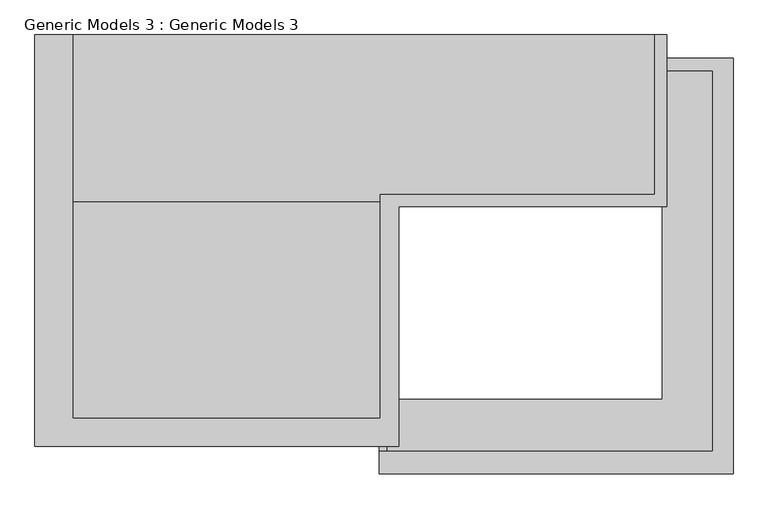
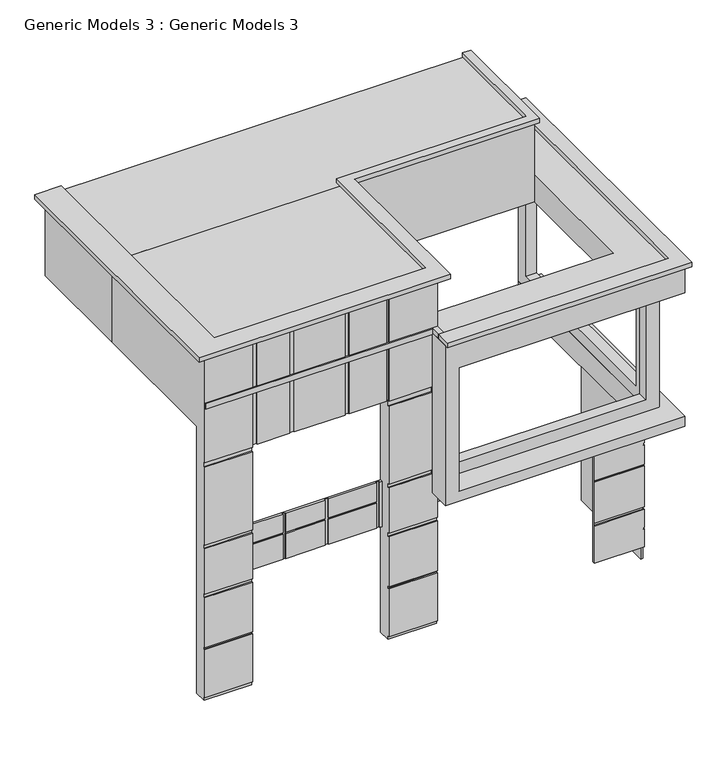
"""IFC4 building model written with IfcOpenShell, lengths in millimetres: proxy geometry, Generic Models 3 : Generic Models 3."""

from ifc_helpers import new_model, si_unit, frame, origin, place, context, project, spatial, polyline, outline, extrude, faceted_brep, source, transform, mapped, element, save


def generic_models_3_generic_models_3_1ac72cdd(model_context):
    return source(origin(), model_context, "Body", "SolidModel", [
        faceted_brep([(-5562.3530968, -13017.658307, 304.8), (-5562.3530968, -12966.858307, 304.8), (-5562.3530968, -12966.858307, 0.0), (-5562.3530968, -12279.4426078, 0.0), (-5562.3530968, -12279.4426078, 707.2361937), (-5562.3530968, -13017.658307, 707.2361937), (-5562.3530968, -13017.658307, 2147.6565444), (-5562.3530968, -13017.658307, 1217.4178641), (-5562.3530968, -12242.958307, 1217.4178641), (-5562.3530968, -12242.958307, 2148.7323728), (-5562.3530968, -12992.258307, 2148.7323728), (-5562.3530968, -12992.258307, 2147.6565444), (-5562.3530968, -12992.258307, 1150.8363185), (-5562.3530968, -13017.658307, 1150.8363185), (-5562.3530968, -13017.658307, 744.9879539), (-5562.3530968, -12242.958307, 744.9879539), (-5562.3530968, -12242.958307, 1148.7718933), (-5562.3530968, -12992.258307, 1148.7718933), (-5562.3530968, -11633.358307, 2630.7756431), (-5562.3530968, -11633.358307, 2189.781496), (-5562.3530968, -10744.358307, 2189.781496), (-5562.3530968, -10744.358307, 2630.7756431), (-5562.3530968, -11633.358307, 1148.7718933), (-5562.3530968, -11633.358307, 744.9879539), (-5562.3530968, -10744.358307, 744.9879539), (-5562.3530968, -10744.358307, 1148.7718933), (-5562.3530968, -11633.358307, 2148.7323728), (-5562.3530968, -11633.358307, 1217.4178641), (-5562.3530968, -10744.358307, 1217.4178641), (-5562.3530968, -10744.358307, 2148.7323728), (-5562.3530968, -12242.958307, 2189.781496), (-5562.3530968, -12242.958307, 2630.7756431), (-5562.3530968, -13017.658307, 2630.7756431), (-5562.3530968, -13017.658307, 2189.781496), (-5562.3530968, -10744.358307, 0.0), (-5562.3530968, -10744.358307, 707.2361937), (-5562.3530968, -11584.7454289, 707.2361937), (-5562.3530968, -11584.7454289, 0.0), (-5562.3530968, -10744.358307, 2670.8659469), (-5562.3530968, -10744.358307, 3048.0), (-5562.3530968, -11633.358307, 3048.0), (-5562.3530968, -11633.358307, 2670.8659469), (-5562.3530968, -13017.658307, 3048.0), (-5562.3530968, -13017.658307, 2670.8659469), (-5562.3530968, -12242.958307, 2670.8659469), (-5562.3530968, -12242.958307, 3048.0), (-5562.3530968, -12242.958307, 0.0), (-5562.3530968, -11633.358307, 0.0), (-5562.3530968, -11633.358307, 707.2361937), (-5562.3530968, -12242.958307, 707.2361937), (-5562.3530968, -11672.0594166, 3048.0), (-5562.3530968, -12209.5923832, 3048.0), (-5562.3530968, -12209.5923832, 2670.8659469), (-5562.3530968, -11672.0594166, 2670.8659469), (-5613.1530968, -12966.858307, 3048.0), (-5613.1530968, -10744.358307, 3048.0), (-5613.1530968, -10744.358307, 0.0), (-5613.1530968, -12966.858307, 0.0), (-5613.1530968, -12966.858307, 304.8), (-5613.1530968, -11633.358307, 2630.7756431), (-5613.1530968, -12242.958307, 2630.7756431), (-5613.1530968, -12242.958307, 744.9879539), (-5613.1530968, -11633.358307, 744.9879539), (-5587.7530968, -11584.7454289, 0.0), (-5587.7530968, -11633.358307, 0.0), (-5587.7530968, -12242.958307, 0.0), (-5587.7530968, -12279.4426078, 0.0), (-5587.7530968, -12242.958307, 2630.7756431), (-5587.7530968, -12242.958307, 2189.781496), (-5587.7530968, -12242.958307, 2148.7323728), (-5587.7530968, -12242.958307, 1217.4178641), (-5587.7530968, -12242.958307, 1148.7718933), (-5587.7530968, -12242.958307, 744.9879539), (-6641.8530968, -12966.858307, 3048.0), (-6641.8530968, -13017.658307, 3048.0), (-5587.7530968, -12242.958307, 3048.0), (-5587.7530968, -12209.5923832, 3048.0), (-5587.7530968, -11672.0594166, 3048.0), (-5587.7530968, -11633.358307, 3048.0), (-5587.7530968, -11633.358307, 2630.7756431), (-5587.7530968, -10744.358307, 2670.8659469), (-5587.7530968, -10744.358307, 2630.7756431), (-5587.7530968, -10744.358307, 2189.781496), (-5587.7530968, -10744.358307, 2148.7323728), (-5587.7530968, -10744.358307, 1217.4178641), (-5587.7530968, -10744.358307, 1148.7718933), (-5587.7530968, -10744.358307, 744.9879539), (-5587.7530968, -10744.358307, 707.2361937), (-5587.7530968, -11633.358307, 744.9879539), (-5587.7530968, -11633.358307, 1148.7718933), (-5587.7530968, -11633.358307, 1217.4178641), (-5587.7530968, -11633.358307, 2148.7323728), (-5587.7530968, -11633.358307, 2189.781496), (-6641.8530968, -13017.658307, 2189.781496), (-5587.7530968, -13017.658307, 2630.7756431), (-5587.7530968, -13017.658307, 2670.8659469), (-6641.8530968, -13017.658307, 304.8), (-5587.7530968, -13017.658307, 707.2361937), (-5587.7530968, -13017.658307, 744.9879539), (-6641.8530968, -13017.658307, 1150.8363185), (-6641.8530968, -13017.658307, 2147.6565444), (-6641.8530968, -13017.658307, 1217.4178641), (-6641.8530968, -12966.858307, 304.8), (-6641.8530968, -12992.258307, 1150.8363185), (-6641.8530968, -12992.258307, 1217.4178641), (-6641.8530968, -12992.258307, 2147.6565444), (-6641.8530968, -12992.258307, 2189.781496), (-5587.7530968, -12992.258307, 1150.8363185), (-5587.7530968, -12992.258307, 1217.4178641), (-5587.7530968, -12992.258307, 2148.7323728), (-5587.7530968, -12992.258307, 2189.781496), (-5587.7530968, -12992.258307, 1148.7718933), (-5587.7530968, -12279.4426078, 707.2361937), (-5587.7530968, -12242.958307, 707.2361937), (-5587.7530968, -11633.358307, 707.2361937), (-5587.7530968, -11584.7454289, 707.2361937), (-5587.7530968, -11672.0594166, 2670.8659469), (-5587.7530968, -12209.5923832, 2670.8659469), (-5587.7530968, -12242.958307, 2670.8659469), (-5587.7530968, -11633.358307, 2670.8659469)], [[[0, 1, 2, 3, 4, 5]], [[6, 7, 8, 9, 10, 11]], [[12, 13, 14, 15, 16, 17]], [[18, 19, 20, 21]], [[22, 23, 24, 25]], [[26, 27, 28, 29]], [[30, 31, 32, 33]], [[34, 35, 36, 37]], [[38, 39, 40, 41]], [[42, 43, 44, 45]], [[46, 47, 48, 49]], [[50, 51, 52, 53]], [[54, 55, 56, 57, 58], [59, 60, 61, 62]], [[57, 2, 1, 58]], [[2, 57, 56, 34, 37, 63, 64, 47, 46, 65, 66, 3]], [[61, 60, 67, 31, 30, 68, 69, 9, 8, 70, 71, 16, 15, 72]], [[55, 54, 73, 74, 42, 45, 75, 76, 51, 50, 77, 78, 40, 39]], [[60, 59, 79, 67]], [[55, 39, 38, 80, 81, 21, 20, 82, 83, 29, 28, 84, 85, 25, 24, 86, 87, 35, 34, 56]], [[59, 62, 88, 23, 22, 89, 90, 27, 26, 91, 92, 19, 18, 79]], [[62, 61, 72, 88]], [[42, 74, 93, 33, 32, 94, 95, 43]], [[96, 0, 5, 97, 98, 14, 13, 99]], [[100, 101, 7, 6]], [[102, 73, 54, 58]], [[73, 102, 96, 99, 103, 104, 101, 100, 105, 106, 93, 74]], [[0, 96, 102, 58, 1]], [[104, 103, 107, 108]], [[105, 11, 10, 109, 110, 106]], [[11, 105, 100, 6]], [[33, 93, 106, 110, 68, 30]], [[13, 12, 107, 103, 99]], [[7, 101, 104, 108, 70, 8]], [[68, 110, 109, 69]], [[70, 108, 107, 111, 71]], [[82, 92, 91, 83]], [[84, 90, 89, 85]], [[72, 98, 97, 112, 66, 65, 113, 114, 64, 63, 115, 87, 86, 88]], [[77, 116, 117, 76, 75, 118, 95, 94, 67, 79, 81, 80, 119, 78]], [[69, 109, 10, 9]], [[71, 111, 17, 16]], [[17, 111, 107, 12]], [[83, 91, 26, 29]], [[92, 82, 20, 19]], [[85, 89, 22, 25]], [[90, 84, 28, 27]], [[49, 48, 114, 113]], [[35, 87, 115, 36]], [[97, 5, 4, 112]], [[98, 72, 15, 14]], [[88, 86, 24, 23]], [[53, 52, 117, 116]], [[80, 38, 41, 119]], [[43, 95, 118, 44]], [[67, 94, 32, 31]], [[81, 79, 18, 21]], [[113, 65, 46, 49]], [[66, 112, 4, 3]], [[115, 63, 37, 36]], [[64, 114, 48, 47]], [[76, 117, 52, 51]], [[118, 75, 45, 44]], [[78, 119, 41, 40]], [[116, 77, 50, 53]]]),
        extrude(outline(polyline([(-10299.4530968, -13297.058307), (-15214.3530968, -13297.058307), (-15214.3530968, -13271.658307), (-10299.4530968, -13271.658307), (-10299.4530968, -13297.058307)])), frame((0.0, 0.0, 6988.8180197), z_axis=(0.0, 0.0, 1.0), x_axis=(1.0, 0.0, 0.0)), (0.0, 0.0, 1.0), 123.1819803),
        extrude(outline(polyline([(-5016.2530968, -13845.289875), (-10299.4530968, -13845.289875), (-10299.4530968, -13513.2632996), (-5320.7863052, -13513.2632996), (-5320.7863052, -7825.1949722), (-6070.3530968, -7825.1949722), (-6070.3530968, -7641.8252058), (-5016.2530968, -7641.8252058), (-5016.2530968, -13845.289875)])), frame((0.0, 0.0, 7010.4), z_axis=(0.0, 0.0, 1.0), x_axis=(1.0, 0.0, 0.0)), (0.0, 0.0, 1.0), 101.6),
        extrude(outline(polyline([(-10185.1530968, -13513.2632996), (-10299.4530968, -13513.2632996), (-10299.4530968, -13271.658307), (-10185.1530968, -13271.658307), (-10185.1530968, -13513.2632996)])), frame((0.0, 0.0, 7010.4), z_axis=(0.0, 0.0, 1.0), x_axis=(1.0, 0.0, 0.0)), (0.0, 0.0, 1.0), 101.6),
        extrude(outline(polyline([(-15436.9164492, -7289.958307), (-14871.4530968, -7289.958307), (-14871.4530968, -13017.658307), (-10285.554919, -13017.658307), (-10285.554919, -9672.4992532), (-6185.8200713, -9672.4992532), (-6185.8200713, -7289.958307), (-6006.8530968, -7289.958307), (-6006.8530968, -9854.918289), (-10002.8085028, -9854.918289), (-10002.8085028, -13437.0410181), (-15436.9164492, -13437.0410181), (-15436.9164492, -7289.958307)])), frame((0.0, 0.0, 8229.6), z_axis=(0.0, 0.0, 1.0), x_axis=(1.0, 0.0, 0.0)), (0.0, 0.0, 1.0), 101.6),
        extrude(outline(polyline([(-6070.3530968, -9781.0408857), (-15214.3530968, -9781.0408857), (-15214.3530968, -7289.958307), (-6070.3530968, -7289.958307), (-6070.3530968, -9781.0408857)])), frame((0.0, 0.0, 6400.8), z_axis=(0.0, 0.0, 1.0), x_axis=(1.0, 0.0, 0.0)), (0.0, 0.0, 1.0), 1828.8),
        faceted_brep([(-5384.1292606, -13043.058307, 6400.8), (-5384.1292606, -13043.058307, 3581.4), (-5384.5530968, -13043.058307, 3581.4), (-5384.5530968, -13043.058307, 6400.8), (-10002.8085028, -13043.058307, 3581.4), (-10002.8085028, -13043.058307, 6400.8), (-5613.1530968, -13043.058307, 6400.8), (-5613.1530968, -13043.058307, 3581.4), (-5676.6530968, -13043.058307, 3851.8605085), (-5676.6530968, -13043.058307, 6146.8), (-9740.6530968, -13043.058307, 6146.8), (-9740.6530968, -13043.058307, 3851.8605085), (-5384.1292606, -13271.658307, 6400.8), (-10002.8085028, -13271.658307, 6400.8), (-10002.8085028, -13271.658307, 3581.4), (-5384.1292606, -13271.658307, 3581.4), (-5676.6530968, -13271.658307, 6146.8), (-5676.6530968, -13271.658307, 3851.8605085), (-9740.6530968, -13271.658307, 3851.8605085), (-9740.6530968, -13271.658307, 6146.8), (-5613.1530968, -8394.858307, 3581.4), (-5384.5530968, -8394.858307, 3581.4), (-5384.5530968, -8394.858307, 6400.8), (-5613.1530968, -8394.858307, 6400.8), (-5384.5530968, -8674.258307, 6146.8), (-5384.5530968, -8674.258307, 3860.8), (-5384.5530968, -12789.058307, 3860.8), (-5384.5530968, -12789.058307, 6146.8), (-5613.1530968, -8674.258307, 3860.8), (-5613.1530968, -8674.258307, 6146.8), (-5613.1530968, -12789.058307, 6146.8), (-5613.1530968, -12789.058307, 3860.8)], [[[0, 1, 2, 3]], [[4, 5, 6, 7], [8, 9, 10, 11]], [[12, 13, 14, 15], [16, 17, 18, 19]], [[1, 0, 12, 15]], [[15, 14, 4, 7, 20, 21, 2, 1]], [[5, 4, 14, 13]], [[13, 12, 0, 3, 22, 23, 6, 5]], [[16, 9, 8, 17]], [[17, 8, 11, 18]], [[18, 11, 10, 19]], [[9, 16, 19, 10]], [[22, 3, 2, 21], [24, 25, 26, 27]], [[23, 20, 7, 6], [28, 29, 30, 31]], [[22, 21, 20, 23]], [[24, 29, 28, 25]], [[25, 28, 31, 26]], [[26, 31, 30, 27]], [[29, 24, 27, 30]]]),
        faceted_brep([(-5117.8530968, -8394.858307, 3581.4), (-5613.1530968, -8394.858307, 3581.4), (-5613.1530968, -12966.858307, 3581.4), (-10299.4530968, -12966.858307, 3581.4), (-10299.4530968, -13271.658307, 3581.4), (-10002.8085028, -13271.658307, 3581.4), (-10002.8085028, -13766.185809, 3581.4), (-5117.8530968, -13766.185809, 3581.4), (-5117.8530968, -13766.185809, 3352.8), (-10299.4530968, -13766.185809, 3352.8), (-10299.4530968, -12966.858307, 3352.8), (-10185.1530968, -12966.858307, 3352.8), (-10185.1530968, -13195.458307, 3352.8), (-5384.5530968, -13195.458307, 3352.8), (-5384.5530968, -8394.858307, 3352.8), (-5117.8530968, -8394.858307, 3352.8), (-5613.1530968, -12966.858307, 3048.0), (-10185.1530968, -12966.858307, 3048.0), (-10299.4530968, -13766.185809, 7010.4), (-10299.4530968, -13271.658307, 7010.4), (-10002.8085028, -13766.185809, 6400.8), (-5117.8530968, -13766.185809, 6400.8), (-5117.8530968, -13766.185809, 7010.4), (-5384.5530968, -8394.858307, 3048.0), (-5613.1530968, -8394.858307, 3048.0), (-5384.5530968, -13195.458307, 3048.0), (-10185.1530968, -13195.458307, 3048.0), (-5117.8530968, -7709.058307, 7010.4), (-6070.3530968, -7709.058307, 7010.4), (-6070.3530968, -12738.258307, 7010.4), (-10185.1530968, -12738.258307, 7010.4), (-10185.1530968, -13271.658307, 7010.4), (-10185.1530968, -13271.658307, 6400.8), (-10002.8085028, -13271.658307, 6400.8), (-10185.1530968, -12738.258307, 6400.8), (-6070.3530968, -12738.258307, 6400.8), (-6070.3530968, -7709.058307, 6400.8), (-5117.8530968, -7709.058307, 6400.8)], [[[0, 1, 2, 3, 4, 5, 6, 7]], [[8, 9, 10, 11, 12, 13, 14, 15]], [[7, 8, 15, 0]], [[10, 3, 2, 16, 17, 11]], [[10, 9, 18, 19, 4, 3]], [[9, 8, 7, 6, 20, 21, 22, 18]], [[1, 0, 15, 14, 23, 24]], [[2, 1, 24, 16]], [[23, 14, 13, 25]], [[16, 24, 23, 25, 26, 17]], [[12, 26, 25, 13]], [[26, 12, 11, 17]], [[19, 18, 22, 27, 28, 29, 30, 31]], [[4, 19, 31, 32, 33, 5]], [[6, 5, 33, 20]], [[21, 20, 33, 32, 34, 35, 36, 37]], [[27, 22, 21, 37]], [[34, 30, 29, 35]], [[30, 34, 32, 31]], [[28, 27, 37, 36]], [[29, 28, 36, 35]]]),
        faceted_brep([(-15214.3530968, -13271.658307, 8229.6), (-15214.3530968, -13271.658307, 5748.0360394), (-14185.6530968, -13271.658307, 5748.0360394), (-14185.6530968, -13271.658307, 8229.6), (-14082.3684215, -13271.658307, 5780.2418911), (-13378.2700012, -13271.658307, 5780.2418911), (-13378.2700012, -13271.658307, 8229.6), (-14082.3684215, -13271.658307, 8229.6), (-13280.9266618, -13271.658307, 5780.2418911), (-12184.1917045, -13271.658307, 5780.2418911), (-12184.1917045, -13271.658307, 8229.6), (-13280.9266618, -13271.658307, 8229.6), (-12099.827477, -13271.658307, 5780.2418911), (-11290.0530968, -13271.658307, 5780.2418911), (-11290.0530968, -13271.658307, 8229.6), (-12099.827477, -13271.658307, 8229.6), (-10185.1530968, -13271.658307, 8229.6), (-11233.851605, -13271.658307, 8229.6), (-11233.851605, -13271.658307, 5767.0860394), (-10299.4530968, -13271.658307, 5767.0860394), (-10299.4530968, -13271.658307, 5646.4360394), (-11233.851605, -13271.658307, 5646.4360394), (-11233.851605, -13271.658307, 3866.4235575), (-10299.4530968, -13271.658307, 3866.4235575), (-10299.4530968, -13271.658307, 3783.7672722), (-11233.851605, -13271.658307, 3783.7672722), (-11233.851605, -13271.658307, 2744.8217298), (-10185.1530968, -13271.658307, 2744.8217298), (-14185.6530968, -13271.658307, 5646.4360394), (-15214.3530968, -13271.658307, 5646.4360394), (-15214.3530968, -13271.658307, 3866.4235575), (-14185.6530968, -13271.658307, 3866.4235575), (-14185.6530968, -13271.658307, 2744.8217298), (-14185.6530968, -13271.658307, 3783.7672722), (-15214.3530968, -13271.658307, 3783.7672722), (-15214.3530968, -13271.658307, 2744.8217298), (-14185.6530968, -13271.658307, 1524.8108649), (-14185.6530968, -13271.658307, 2666.5766837), (-15214.3530968, -13271.658307, 2666.5766837), (-15214.3530968, -13271.658307, 1524.8108649), (-14185.6530968, -13271.658307, 382.6097323), (-14185.6530968, -13271.658307, 1479.6035006), (-15214.3530968, -13271.658307, 1479.6035006), (-15214.3530968, -13271.658307, 382.6097323), (-10185.1530968, -13271.658307, 382.6097323), (-10185.1530968, -13271.658307, 1479.6035006), (-11233.851605, -13271.658307, 1479.6035006), (-11233.851605, -13271.658307, 382.6097323), (-10185.1530968, -13271.658307, 1524.0), (-10185.1530968, -13271.658307, 2666.5766837), (-11233.851605, -13271.658307, 2666.5766837), (-11233.851605, -13271.658307, 1524.0), (-15214.3530968, -12966.858307, 6400.8), (-10185.1530968, -12966.858307, 6400.8), (-10185.1530968, -12966.858307, 304.8), (-11233.851605, -12966.858307, 304.8), (-11233.851605, -12966.858307, 2744.8217298), (-14185.6530968, -12966.858307, 2744.8217298), (-14185.6530968, -12966.858307, 304.8), (-15214.3530968, -12966.858307, 304.8), (-11233.851605, -12966.858307, 5780.2418911), (-14185.6530968, -12966.858307, 5780.2418911), (-14185.6530968, -12966.858307, 3783.7672722), (-11233.851605, -12966.858307, 3783.7672722), (-15214.3530968, -9781.0408857, 8229.6), (-15214.3530968, -9781.0408857, 6400.8), (-15214.3530968, -13246.258307, 304.8), (-15214.3530968, -13246.258307, 382.6097323), (-15214.3530968, -13246.258307, 1479.6035006), (-15214.3530968, -13246.258307, 1524.8108649), (-15214.3530968, -13246.258307, 2666.5766837), (-15214.3530968, -13246.258307, 2744.8217298), (-15214.3530968, -13246.258307, 3783.7672722), (-15214.3530968, -13246.258307, 3866.4235575), (-15214.3530968, -13246.258307, 5646.4360394), (-15214.3530968, -13246.258307, 5748.0360394), (-11233.851605, -13246.258307, 5780.2418911), (-11290.0530968, -13246.258307, 5780.2418911), (-12099.827477, -13246.258307, 5780.2418911), (-12184.1917045, -13246.258307, 5780.2418911), (-13280.9266618, -13246.258307, 5780.2418911), (-13378.2700012, -13246.258307, 5780.2418911), (-14082.3684215, -13246.258307, 5780.2418911), (-14185.6530968, -13246.258307, 5780.2418911), (-10185.1530968, -9781.0408857, 8229.6), (-10185.1530968, -13246.258307, 2744.8217298), (-10185.1530968, -13246.258307, 2666.5766837), (-10185.1530968, -13246.258307, 1524.0), (-10185.1530968, -13246.258307, 1479.6035006), (-10185.1530968, -13246.258307, 382.6097323), (-10185.1530968, -13246.258307, 304.8), (-10185.1530968, -9781.0408857, 6400.8), (-14185.6530968, -13246.258307, 8229.6), (-14082.3684215, -13246.258307, 8229.6), (-13378.2700012, -13246.258307, 8229.6), (-13280.9266618, -13246.258307, 8229.6), (-12184.1917045, -13246.258307, 8229.6), (-12099.827477, -13246.258307, 8229.6), (-11290.0530968, -13246.258307, 8229.6), (-11233.851605, -13246.258307, 8229.6), (-14185.6530968, -13246.258307, 304.8), (-14185.6530968, -13246.258307, 5748.0360394), (-14185.6530968, -13246.258307, 5646.4360394), (-14185.6530968, -13246.258307, 3866.4235575), (-14185.6530968, -13246.258307, 3783.7672722), (-14185.6530968, -13246.258307, 2744.8217298), (-14185.6530968, -13246.258307, 2666.5766837), (-14185.6530968, -13246.258307, 1524.8108649), (-14185.6530968, -13246.258307, 1479.6035006), (-14185.6530968, -13246.258307, 382.6097323), (-14185.6530968, -13017.658307, 2744.8217298), (-14185.6530968, -13017.658307, 3316.5628288), (-14185.6530968, -12992.258307, 3316.5628288), (-14185.6530968, -12992.258307, 3352.8), (-14185.6530968, -13017.658307, 3352.8), (-14185.6530968, -13017.658307, 3783.7672722), (-11233.851605, -13017.658307, 3783.7672722), (-11233.851605, -13017.658307, 2744.8217298), (-11233.851605, -13246.258307, 304.8), (-11233.851605, -13246.258307, 382.6097323), (-11233.851605, -13246.258307, 1479.6035006), (-11233.851605, -13246.258307, 1524.0), (-11233.851605, -13246.258307, 2666.5766837), (-11233.851605, -13246.258307, 2744.8217298), (-11233.851605, -13246.258307, 3783.7672722), (-11233.851605, -13246.258307, 3866.4235575), (-11233.851605, -13246.258307, 5646.4360394), (-11233.851605, -13246.258307, 5767.0860394), (-11290.0530968, -13017.658307, 3783.7672722), (-11290.0530968, -13017.658307, 3352.8), (-11290.0530968, -13017.658307, 3316.5628288), (-11290.0530968, -13017.658307, 2744.8217298), (-13379.2030968, -13017.658307, 3783.7672722), (-13379.2030968, -13017.658307, 3352.8), (-12464.8030968, -13017.658307, 3783.7672722), (-13326.1879226, -13017.658307, 3783.7672722), (-13326.1879226, -13017.658307, 3352.8), (-12464.8030968, -13017.658307, 3352.8), (-13379.2030968, -13017.658307, 2744.8217298), (-13379.2030968, -13017.658307, 3316.5628288), (-13326.1879226, -13017.658307, 2744.8217298), (-12464.8030968, -13017.658307, 2744.8217298), (-12464.8030968, -13017.658307, 3316.5628288), (-13326.1879226, -13017.658307, 3316.5628288), (-11353.5530968, -13017.658307, 3783.7672722), (-12392.6457873, -13017.658307, 3783.7672722), (-12392.6457873, -13017.658307, 3352.8), (-11353.5530968, -13017.658307, 3352.8), (-12392.6457873, -13017.658307, 2744.8217298), (-11353.5530968, -13017.658307, 2744.8217298), (-11353.5530968, -13017.658307, 3316.5628288), (-12392.6457873, -13017.658307, 3316.5628288), (-13379.2030968, -12992.258307, 3783.7672722), (-13326.1879226, -12992.258307, 3783.7672722), (-12464.8030968, -12992.258307, 3783.7672722), (-12392.6457873, -12992.258307, 3783.7672722), (-11353.5530968, -12992.258307, 3783.7672722), (-11290.0530968, -12992.258307, 3783.7672722), (-11290.0530968, -12992.258307, 2744.8217298), (-11353.5530968, -12992.258307, 2744.8217298), (-12392.6457873, -12992.258307, 2744.8217298), (-12464.8030968, -12992.258307, 2744.8217298), (-13326.1879226, -12992.258307, 2744.8217298), (-13379.2030968, -12992.258307, 2744.8217298), (-10299.4530968, -13246.258307, 5646.4360394), (-10299.4530968, -13246.258307, 5767.0860394), (-10299.4530968, -13246.258307, 3783.7672722), (-10299.4530968, -13246.258307, 3866.4235575), (-13379.2030968, -12992.258307, 3352.8), (-13379.2030968, -12992.258307, 3316.5628288), (-13326.1879226, -12992.258307, 3316.5628288), (-12464.8030968, -12992.258307, 3316.5628288), (-12392.6457873, -12992.258307, 3316.5628288), (-11353.5530968, -12992.258307, 3316.5628288), (-11353.5530968, -12992.258307, 3352.8), (-12392.6457873, -12992.258307, 3352.8), (-12464.8030968, -12992.258307, 3352.8), (-13326.1879226, -12992.258307, 3352.8)], [[[0, 1, 2, 3]], [[4, 5, 6, 7]], [[8, 9, 10, 11]], [[12, 13, 14, 15]], [[16, 17, 18, 19, 20, 21, 22, 23, 24, 25, 26, 27]], [[28, 29, 30, 31]], [[32, 33, 34, 35]], [[36, 37, 38, 39]], [[40, 41, 42, 43]], [[44, 45, 46, 47]], [[48, 49, 50, 51]], [[52, 53, 54, 55, 56, 57, 58, 59], [60, 61, 62, 63]], [[0, 64, 65, 52, 59, 66, 67, 43, 42, 68, 69, 39, 38, 70, 71, 35, 34, 72, 73, 30, 29, 74, 75, 1]], [[61, 60, 76, 77, 13, 12, 78, 79, 9, 8, 80, 81, 5, 4, 82, 83]], [[84, 16, 27, 85, 86, 49, 48, 87, 88, 45, 44, 89, 90, 54, 53, 91]], [[16, 84, 64, 0, 3, 92, 93, 7, 6, 94, 95, 11, 10, 96, 97, 15, 14, 98, 99, 17]], [[65, 91, 53, 52]], [[64, 84, 91, 65]], [[59, 58, 100, 66]], [[62, 61, 83, 92, 3, 2, 101, 102, 28, 31, 103, 104, 33, 32, 105, 106, 37, 36, 107, 108, 41, 40, 109, 100, 58, 57, 110, 111, 112, 113, 114, 115]], [[60, 63, 116, 117, 56, 55, 118, 119, 47, 46, 120, 121, 51, 50, 122, 123, 26, 25, 124, 125, 22, 21, 126, 127, 18, 17, 99, 76]], [[55, 54, 90, 118]], [[117, 116, 128, 129, 130, 131]], [[132, 115, 114, 133]], [[134, 135, 136, 137]], [[110, 138, 139, 111]], [[140, 141, 142, 143]], [[144, 145, 146, 147]], [[148, 149, 150, 151]], [[63, 62, 115, 132, 152, 153, 135, 134, 154, 155, 145, 144, 156, 157, 128, 116]], [[57, 56, 117, 131, 158, 159, 149, 148, 160, 161, 141, 140, 162, 163, 138, 110]], [[76, 99, 98, 77]], [[101, 75, 74, 102]], [[82, 93, 92, 83]], [[80, 95, 94, 81]], [[78, 97, 96, 79]], [[126, 164, 165, 127]], [[102, 74, 29, 28]], [[75, 101, 2, 1]], [[93, 82, 4, 7]], [[81, 94, 6, 5]], [[95, 80, 8, 11]], [[79, 96, 10, 9]], [[97, 78, 12, 15]], [[77, 98, 14, 13]], [[127, 165, 19, 18]], [[165, 164, 20, 19]], [[164, 126, 21, 20]], [[72, 104, 103, 73]], [[166, 167, 125, 124]], [[70, 106, 105, 71]], [[85, 123, 122, 86]], [[109, 67, 66, 100]], [[68, 108, 107, 69]], [[89, 119, 118, 90]], [[87, 121, 120, 88]], [[73, 103, 31, 30]], [[104, 72, 34, 33]], [[166, 124, 25, 24]], [[125, 167, 23, 22]], [[167, 166, 24, 23]], [[71, 105, 32, 35]], [[106, 70, 38, 37]], [[86, 122, 50, 49]], [[123, 85, 27, 26]], [[67, 109, 40, 43]], [[69, 107, 36, 39]], [[108, 68, 42, 41]], [[119, 89, 44, 47]], [[88, 120, 46, 45]], [[121, 87, 48, 51]], [[153, 152, 168, 113, 112, 169, 163, 162, 170, 171, 161, 160, 172, 173, 159, 158, 157, 156, 174, 175, 155, 154, 176, 177]], [[135, 153, 177, 136]], [[162, 140, 143, 170]], [[152, 132, 133, 168]], [[138, 163, 169, 139]], [[145, 155, 175, 146]], [[160, 148, 151, 172]], [[154, 134, 137, 176]], [[141, 161, 171, 142]], [[128, 157, 158, 131, 130, 129]], [[156, 144, 147, 174]], [[149, 159, 173, 150]], [[112, 111, 139, 169]], [[171, 170, 143, 142]], [[173, 172, 151, 150]], [[114, 113, 168, 133]], [[175, 174, 147, 146]], [[177, 176, 137, 136]]]),
    ])


if __name__ == "__main__":
    model = new_model("IFC4")
    model_context = context("Model", 3, world=origin())
    ifc_project = project(units=[si_unit("LENGTHUNIT", "METRE", prefix="MILLI")], contexts=[model_context])
    site = spatial("IfcSite", under=ifc_project)
    building = spatial("IfcBuilding", under=site)
    placement = place(None, origin())
    generic_models_3_generic_models_3_shape = generic_models_3_generic_models_3_1ac72cdd(model_context)
    element("IfcBuildingElementProxy", 1, Name="Generic Models 3 : Generic Models 3", ObjectType="Generic Models 3 : Generic Models 3", at=placement, inside=building, context=model_context, shape_type="MappedRepresentation", body=[
        mapped(generic_models_3_generic_models_3_shape, transform((0.0, 0.0, 0.0), x_axis=(1.0, 0.0, 0.0), y_axis=(0.0, 1.0, 0.0), z_axis=(0.0, 0.0, 1.0))),
    ])
    save(model, "model.ifc")

# Revit data of these elements
# Element 1 (IfcBuildingElementProxy, "Generic Models 3 : Generic Models 3")
#   Materials on its faces: "Structure, Wood Joist/Rafter Layer, Batt Insulation"
# Materials
#   "Structure, Wood Joist/Rafter Layer, Batt Insulation": class "Wood", colour RGB 127 127 127, transparency 0, Description = "Wood framing, insulated", Cost = 0
